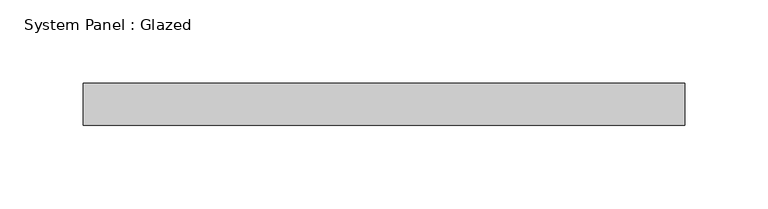
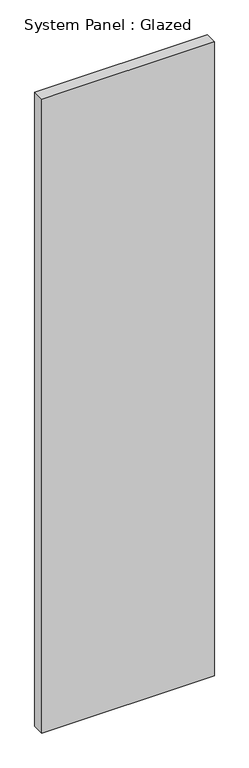
"""IFC4 building model written with IfcOpenShell, lengths in millimetres: plate geometry, System Panel : Glazed."""

from ifc_helpers import new_model, si_unit, origin, origin_with_axes, place, context, project, spatial, polyline, outline, extrude, source, transform, mapped, element, save


def system_panel_glazed_03b7eec7(model_context):
    return source(origin(), model_context, "Body", "SweptSolid", [
        extrude(outline(polyline([(180.975, 19.05), (-180.975, 19.05), (-180.975, 44.45), (180.975, 44.45), (180.975, 19.05)])), origin_with_axes(), (0.0, 0.0, 1.0), 1405.0284144),
    ])


if __name__ == "__main__":
    model = new_model("IFC4")
    model_context = context("Model", 3, world=origin())
    ifc_project = project(units=[si_unit("LENGTHUNIT", "METRE", prefix="MILLI")], contexts=[model_context])
    site = spatial("IfcSite", under=ifc_project)
    building = spatial("IfcBuilding", under=site)
    placement = place(None, origin())
    system_panel_glazed_shape = system_panel_glazed_03b7eec7(model_context)
    element("IfcPlate", 1, ObjectType="System Panel : Glazed", at=placement, inside=building, context=model_context, shape_type="MappedRepresentation", body=[
        mapped(system_panel_glazed_shape, transform((0.0, 0.0, 0.0), x_axis=(1.0, 0.0, 0.0), y_axis=(0.0, 1.0, 0.0), z_axis=(0.0, 0.0, 1.0))),
    ])
    save(model, "model.ifc")

# Revit data of these elements
# Type "System Panel : Glazed"
#   Construction Type Id = "GSP4R"
#   Analytic Construction = "1/8 in Pilkington single glazing"
#   Visual Light Transmittance = 0.9
#   Solar Heat Gain Coefficient = 0.86
#   Heat Transfer Coefficient (U) = 1.18115 BTU/(h·ft²·°F)
#   Define Thermal Properties by = 1
# Element 1 (IfcPlate, "System Panel : Glazed")
#   Materials on its faces: "Glass"
# Materials
#   "Glass": class "Glass", colour RGB 0 128 192, transparency 0.75, Description = "Soda Lime Glass", Cost = 0
